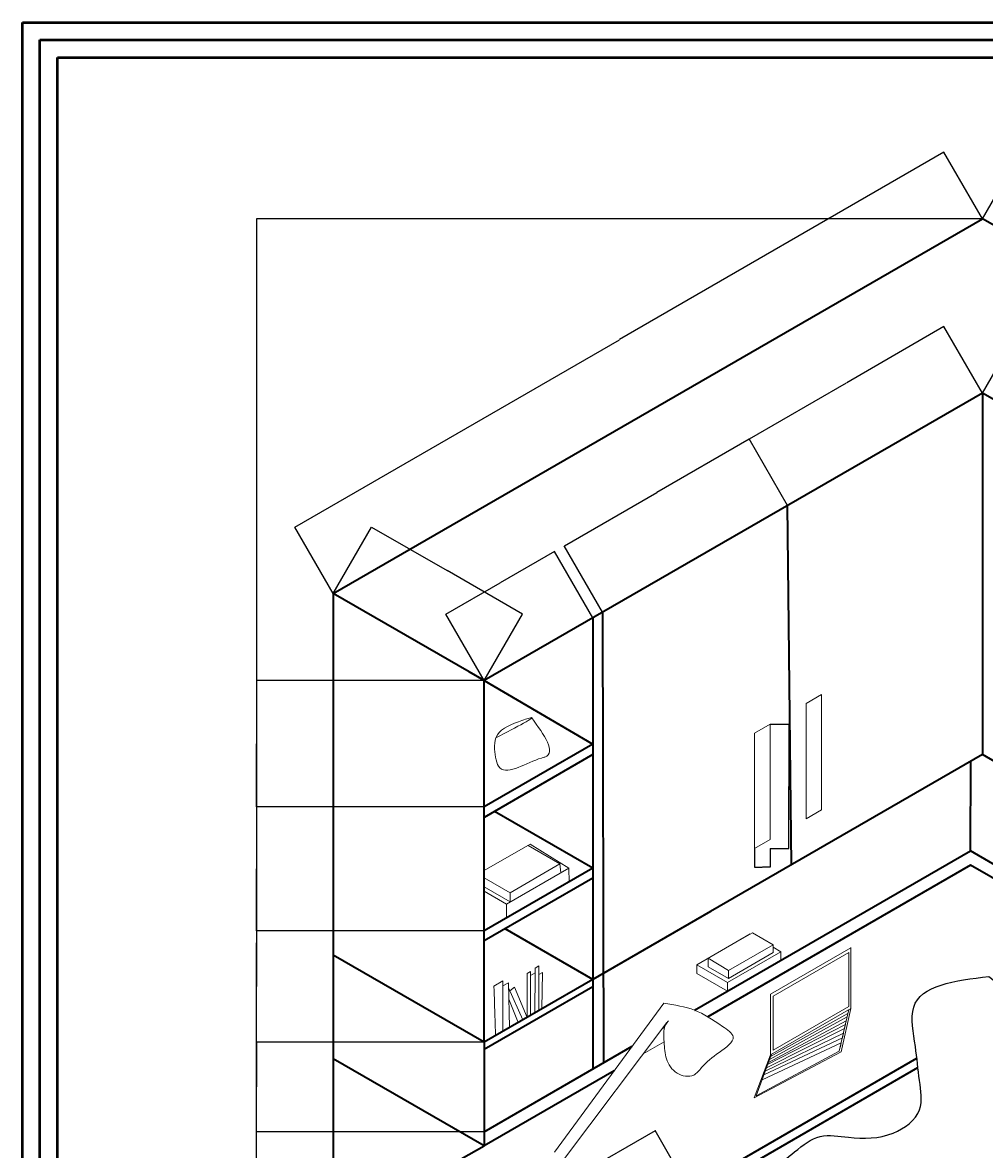
# Model space of a CAD drawing. Units: millimetres. Extents: x -2976 to 8877, y -7187 to 5690.
# Tile 2 of 2: x -2976 to 2542, y -776 to 5690. Entities that reach past the tile are written whole.
import ezdxf

# ---------------------------------------------------------------- set-up
doc = ezdxf.new("R2010")
doc.units = ezdxf.units.MM
doc.header["$MEASUREMENT"] = 0
for name, color, linetype, lineweight in [('A-ANNO-DIMS', 2, 'Continuous', 18), ('A-ANNO-TTLB', 7, 'Continuous', 50), ('A-FURN', 7, 'Continuous', 35), ('A-FURN-ACCS', 3, 'Continuous', 18), ('A-FURN-CHAIR', 4, 'Continuous', 25), ('A-FURN-HDWR', 8, 'Continuous', 18)]:
    doc.layers.add(name, color=color, linetype=linetype, lineweight=lineweight)
doc.styles.get("Standard").update_dxf_attribs({"font": 'arial.ttf'})
doc.dimstyles.get("Standard").update_dxf_attribs({"dimtxt": 0.18, "dimasz": 0.18, "dimexe": 0.18, "dimexo": 0.0625, "dimgap": 0.09, "dimtad": 0, "dimtih": 1, "dimtoh": 1, "dimdec": 0, "dimzin": 0, "dimdsep": 46, "dimtxsty": 'Standard', "dimcen": 0.09, "dimadec": 0, "dimazin": 0, "dimtfac": 1, "dimtdec": 0, "dimtofl": 0, "dimtmove": 0, "dimatfit": 3, "dimfxl": 1, "dimtolj": 1, "dimtzin": 0, "dimarcsym": 0})

# ---------------------------------------------------------------- blocks, each defined once
blk = doc.blocks.new('HANDLE-DOOR-L')
for p, q in [((89.65431383447503, 713.2380158491153), (-0.0001289517056193, 661.4759991724679)), ((89.65431383447503, 51.7624652354541), (89.65431383447503, 713.2380158491153)), ((-0.0001289517058467, 0.0004485588067382), (-0.0001289517058467, 661.4759991724676)), ((-0.0001289517058467, 0.0004485588067382), (89.65431383447503, 51.7624652354541))]:
    blk.add_line(p, q)
blk = doc.blocks.new('*D9')
at = {"layer": 'A-ANNO-DIMS', "color": 0, "lineweight": -2, "transparency": 16777216}
for p, q in [((1313.18315975467, 1663.813910547956), (1420.286294848217, 1663.813910547956)), ((1420.106294848217, 1663.633910547956), (1420.106294848217, 1307.403182837317)), ((1420.106294848217, 950.7563432576469), (1420.106294848217, 1306.987070968286)), ((1313.18315975467, 950.576343257647), (1420.286294848217, 950.576343257647))]:
    blk.add_line(p, q, dxfattribs=at)
at = {"layer": 'A-ANNO-DIMS', "color": 0, "transparency": 16777216}
for points in [[(1420.076294848217, 1663.633910547956), (1420.136294848217, 1663.633910547956), (1420.106294848217, 1663.813910547956)], [(1420.076294848217, 950.7563432576469), (1420.136294848217, 950.7563432576469), (1420.106294848217, 950.576343257647)]]:
    blk.add_solid(points, dxfattribs=at)
at = {"layer": 'Defpoints', "color": 0, "transparency": 16777216}
for p in [(1313.12065975467, 1663.813910547956), (1313.12065975467, 950.576343257647), (1420.106294848217, 950.576343257647)]:
    blk.add_point(p, dxfattribs=at)
at = {"layer": 'A-ANNO-DIMS', "color": 0, "transparency": 16777216, "insert": (1420.106294848217, 1307.195126902801), "char_height": 0.18, "attachment_point": 5}
blk.add_mtext('\\A1;DOOR HANDLE (LEFT) 713 TYP.', dxfattribs=at)
blk = doc.blocks.new('*D10')
at = {"layer": 'A-ANNO-DIMS', "color": 0, "lineweight": -2, "transparency": 16777216}
for p, q in [((1223.466216968489, 950.5138432576465), (1223.466216968489, 843.4107081641002)), ((1313.12065975467, 950.5138432576465), (1313.12065975467, 843.4107081641002)), ((1223.646216968489, 843.5907081641003), (1267.765348320651, 843.5907081641003)), ((1312.94065975467, 843.5907081641003), (1268.821528402507, 843.5907081641003))]:
    blk.add_line(p, q, dxfattribs=at)
at = {"layer": 'A-ANNO-DIMS', "color": 0, "transparency": 16777216}
for points in [[(1223.646216968489, 843.6207081641002), (1223.646216968489, 843.5607081641004), (1223.466216968489, 843.5907081641003)], [(1312.94065975467, 843.6207081641002), (1312.94065975467, 843.5607081641004), (1313.12065975467, 843.5907081641003)]]:
    blk.add_solid(points, dxfattribs=at)
at = {"layer": 'Defpoints', "color": 0, "transparency": 16777216}
for p in [(1223.466216968489, 950.5763432576467), (1313.12065975467, 950.5763432576467), (1223.466216968489, 843.5907081641003)]:
    blk.add_point(p, dxfattribs=at)
at = {"layer": 'A-ANNO-DIMS', "color": 0, "transparency": 16777216, "insert": (1268.293438361579, 843.5907081641003), "char_height": 0.18, "attachment_point": 5}
blk.add_mtext('\\A1;90 TYP.', dxfattribs=at)
blk = doc.blocks.new('*D14')
at = {"layer": 'A-ANNO-DIMS', "color": 0, "lineweight": -2, "transparency": 16777216}
for p, q in [((2530.179259000001, 4564.359981000001), (-1633.847478000003, 4564.359981)), ((-1633.667478000003, 4564.179981), (-1633.667478000002, 411.1110510293304)), ((-1633.667478000001, -3742.321808000003), (-1633.667478000002, 410.7471219706673)), ((-327.7045740000001, -3742.501808000002), (-1633.847478000001, -3742.501808000002))]:
    blk.add_line(p, q, dxfattribs=at)
at = {"layer": 'A-ANNO-DIMS', "color": 0, "transparency": 16777216}
for points in [[(-1633.697478000003, 4564.179981), (-1633.637478000003, 4564.179981), (-1633.667478000003, 4564.359981)], [(-1633.697478000001, -3742.321808000003), (-1633.637478000001, -3742.321808000003), (-1633.667478000001, -3742.501808000002)]]:
    blk.add_solid(points, dxfattribs=at)
at = {"layer": 'Defpoints', "color": 0, "transparency": 16777216}
for p in [(2530.241759000001, 4564.359981000001), (-1633.667478000001, -3742.501808000002), (-327.6420740000001, -3742.501808000002)]:
    blk.add_point(p, dxfattribs=at)
at = {"layer": 'A-ANNO-DIMS', "color": 0, "transparency": 16777216, "insert": (-1633.667478000001, 410.9290864999992), "char_height": 0.18, "attachment_point": 5}
blk.add_mtext('\\A1;8307', dxfattribs=at)
blk = doc.blocks.new('*D16')
at = {"layer": 'A-ANNO-DIMS', "color": 0, "lineweight": -2, "transparency": 16777216}
for p, q in [((-327.7045740000001, 1914.359981000001), (-1633.847478000002, 1914.359981)), ((-1633.667478000002, 1914.179981), (-1633.667478000002, 1552.47832434925)), ((-1633.667478000002, 1190.415931), (-1633.667478000002, 1552.117587650751)), ((-327.7045740000001, 1190.235931), (-1633.847478000001, 1190.235931))]:
    blk.add_line(p, q, dxfattribs=at)
at = {"layer": 'A-ANNO-DIMS', "color": 0, "transparency": 16777216}
for points in [[(-1633.697478000002, 1914.179981), (-1633.637478000002, 1914.179981), (-1633.667478000002, 1914.359981)], [(-1633.697478000001, 1190.415931), (-1633.637478000002, 1190.415931), (-1633.667478000002, 1190.235931)]]:
    blk.add_solid(points, dxfattribs=at)
at = {"layer": 'Defpoints', "color": 0, "transparency": 16777216}
for p in [(-327.6420740000001, 1914.359981000001), (-1633.667478000002, 1190.235931), (-327.6420740000001, 1190.235931)]:
    blk.add_point(p, dxfattribs=at)
at = {"layer": 'A-ANNO-DIMS', "color": 0, "transparency": 16777216, "insert": (-1633.667478000001, 1552.297956), "char_height": 0.18, "attachment_point": 5}
blk.add_mtext('\\A1;724.1', dxfattribs=at)
blk = doc.blocks.new('*D17')
at = {"layer": 'A-ANNO-DIMS', "color": 0, "lineweight": -2, "transparency": 16777216}
for p, q in [((-327.7045740000001, 1190.235931), (-1633.847478000001, 1190.235931)), ((-1633.667478000002, 1190.055931), (-1633.667478000002, 834.1931958492496)), ((-1633.667478000002, 477.9697239999999), (-1633.667478000002, 833.8324591507504)), ((-327.7045740000001, 477.7897240000002), (-1633.847478000001, 477.7897239999999))]:
    blk.add_line(p, q, dxfattribs=at)
at = {"layer": 'A-ANNO-DIMS', "color": 0, "transparency": 16777216}
for points in [[(-1633.697478000002, 1190.055931), (-1633.637478000002, 1190.055931), (-1633.667478000002, 1190.235931)], [(-1633.697478000001, 477.9697239999999), (-1633.637478000002, 477.9697239999999), (-1633.667478000002, 477.7897239999999)]]:
    blk.add_solid(points, dxfattribs=at)
at = {"layer": 'Defpoints', "color": 0, "transparency": 16777216}
for p in [(-327.6420740000001, 1190.235931), (-1633.667478000002, 477.7897239999999), (-327.6420740000001, 477.7897240000002)]:
    blk.add_point(p, dxfattribs=at)
at = {"layer": 'A-ANNO-DIMS', "color": 0, "transparency": 16777216, "insert": (-1633.667478000001, 834.0128275000003), "char_height": 0.18, "attachment_point": 5}
blk.add_mtext('\\A1;712.4', dxfattribs=at)
blk = doc.blocks.new('*D18')
at = {"layer": 'A-ANNO-DIMS', "color": 0, "lineweight": -2, "transparency": 16777216}
for p, q in [((-327.7045740000001, 477.7897240000002), (-1633.847478000002, 477.7897239999999)), ((-1633.667478000002, 477.6097239999999), (-1633.667478000002, 158.9980610293313)), ((-1633.667478000002, -159.9775310000002), (-1633.667478000002, 158.6341319706683)), ((-327.7045740000001, -160.1575310000001), (-1633.847478000002, -160.1575310000002))]:
    blk.add_line(p, q, dxfattribs=at)
at = {"layer": 'A-ANNO-DIMS', "color": 0, "transparency": 16777216}
for points in [[(-1633.697478000002, 477.6097239999999), (-1633.637478000002, 477.6097239999999), (-1633.667478000002, 477.7897239999999)], [(-1633.697478000002, -159.9775310000002), (-1633.637478000002, -159.9775310000002), (-1633.667478000002, -160.1575310000002)]]:
    blk.add_solid(points, dxfattribs=at)
at = {"layer": 'Defpoints', "color": 0, "transparency": 16777216}
for p in [(-327.6420740000001, 477.7897240000002), (-1633.667478000002, -160.1575310000002), (-327.6420740000001, -160.1575310000001)]:
    blk.add_point(p, dxfattribs=at)
at = {"layer": 'A-ANNO-DIMS', "color": 0, "transparency": 16777216, "insert": (-1633.667478000001, 158.8160965000003), "char_height": 0.18, "attachment_point": 5}
blk.add_mtext('\\A1;638', dxfattribs=at)
blk = doc.blocks.new('*D19')
at = {"layer": 'A-ANNO-DIMS', "color": 0, "lineweight": -2, "transparency": 16777216}
for p, q in [((-327.7045740000001, -160.1575310000001), (-1633.847478000002, -160.1575310000002)), ((-1633.667478000002, -160.3375310000003), (-1633.667478000002, -416.6881374706688)), ((-1633.667478000002, -673.4026730000003), (-1633.667478000002, -417.0520665293318)), ((-327.7045740000001, -673.5826730000002), (-1633.847478000001, -673.5826730000003))]:
    blk.add_line(p, q, dxfattribs=at)
at = {"layer": 'A-ANNO-DIMS', "color": 0, "transparency": 16777216}
for points in [[(-1633.697478000002, -160.3375310000003), (-1633.637478000002, -160.3375310000003), (-1633.667478000002, -160.1575310000002)], [(-1633.697478000001, -673.4026730000003), (-1633.637478000002, -673.4026730000003), (-1633.667478000002, -673.5826730000003)]]:
    blk.add_solid(points, dxfattribs=at)
at = {"layer": 'Defpoints', "color": 0, "transparency": 16777216}
for p in [(-327.6420740000001, -160.1575310000001), (-1633.667478000002, -673.5826730000003), (-327.6420740000001, -673.5826730000002)]:
    blk.add_point(p, dxfattribs=at)
at = {"layer": 'A-ANNO-DIMS', "color": 0, "transparency": 16777216, "insert": (-1633.667478000001, -416.8701019999998), "char_height": 0.18, "attachment_point": 5}
blk.add_mtext('\\A1;513.4', dxfattribs=at)
blk = doc.blocks.new('*D24')
at = {"layer": 'A-ANNO-DIMS', "color": 0, "lineweight": -2, "transparency": 16777216}
for p, q in [((652.7837904139722, -667.9703643117301), (52.96397228998472, -1014.276497770886)), ((872.9084249999999, -1048.877415412263), (652.8496749866534, -667.7244797390488)), ((-547.4861894539579, -1360.946560288706), (52.33362867002966, -1014.640426829549)), ((-327.6733239999999, -1742.033611412263), (-547.7320740266391, -1360.880675716025))]:
    blk.add_line(p, q, dxfattribs=at)
at = {"layer": 'A-ANNO-DIMS', "color": 0, "transparency": 16777216}
for points in [[(652.7687904139723, -667.9443835496166), (652.7987904139723, -667.9963450738435), (652.9396749866535, -667.8803643117301)], [(-547.5011894539577, -1360.920579526592), (-547.4711894539579, -1360.972541050819), (-547.6420740266392, -1361.036560288706)]]:
    blk.add_solid(points, dxfattribs=at)
at = {"layer": 'Defpoints', "color": 0, "transparency": 16777216}
for p in [(652.9396749866535, -667.8803643117301), (872.9396749999999, -1048.931542), (-327.6420739999999, -1742.087737999999)]:
    blk.add_point(p, dxfattribs=at)
at = {"layer": 'A-ANNO-DIMS', "color": 0, "transparency": 16777216, "insert": (52.64880048000714, -1014.458462300218), "char_height": 0.18, "attachment_point": 5}
blk.add_mtext('\\A1;1386.3', dxfattribs=at)
blk = doc.blocks.new('*D25')
at = {"layer": 'A-ANNO-DIMS', "color": 0, "lineweight": -2, "transparency": 16777216}
for p, q in [((2310.085874749474, 4945.321158107162), (448.6023127229957, 3870.593122479113)), ((2530.210509, 4564.414107587736), (2310.151759322155, 4945.567042679844)), ((-1413.511592923435, 2795.501157792401), (447.9719691030407, 3870.22919342045)), ((-1193.698728, 2414.414107587737), (-1413.757477496116, 2795.567042365082))]:
    blk.add_line(p, q, dxfattribs=at)
at = {"layer": 'A-ANNO-DIMS', "color": 0, "transparency": 16777216}
for points in [[(2310.070874749474, 4945.347138869276), (2310.100874749474, 4945.295177345049), (2310.241759322155, 4945.411158107162)], [(-1413.526592923435, 2795.527138554515), (-1413.496592923435, 2795.475177030287), (-1413.667477496116, 2795.411157792401)]]:
    blk.add_solid(points, dxfattribs=at)
at = {"layer": 'Defpoints', "color": 0, "transparency": 16777216}
for p in [(2310.241759322155, 4945.411158107162), (2530.241759, 4564.359980999999), (-1193.667478, 2414.359981)]:
    blk.add_point(p, dxfattribs=at)
at = {"layer": 'A-ANNO-DIMS', "color": 0, "transparency": 16777216, "insert": (448.2871409130193, 3870.411157949782), "char_height": 0.18, "attachment_point": 5}
blk.add_mtext('\\A1;4300', dxfattribs=at)
blk = doc.blocks.new('*D26')
at = {"layer": 'A-ANNO-DIMS', "color": 0, "lineweight": -2, "transparency": 16777216}
for p, q in [((2530.273009, 4564.414107587735), (2750.331758610178, 4945.567042562642)), ((2750.397643182859, 4945.321157989961), (5131.496553235272, 3570.593061304077)), ((7513.225594241101, 2195.501158342615), (5132.126684188691, 3570.229255028497)), ((7293.412728999999, 1814.414107587736), (7513.471478813783, 2195.567042915297))]:
    blk.add_line(p, q, dxfattribs=at)
at = {"layer": 'A-ANNO-DIMS', "color": 0, "transparency": 16777216}
for points in [[(2750.412643182859, 4945.347138752074), (2750.382643182859, 4945.295177227848), (2750.241758610178, 4945.411157989961)], [(7513.240594241101, 2195.527139104729), (7513.210594241101, 2195.475177580502), (7513.381478813783, 2195.411158342615)]]:
    blk.add_solid(points, dxfattribs=at)
at = {"layer": 'Defpoints', "color": 0, "transparency": 16777216}
for p in [(2530.241759, 4564.359980999999), (7513.381478813783, 2195.411158342615), (7293.381479, 1814.359981)]:
    blk.add_point(p, dxfattribs=at)
at = {"layer": 'A-ANNO-DIMS', "color": 0, "transparency": 16777216, "insert": (5131.81161871198, 3570.411158166288), "char_height": 0.18, "attachment_point": 5}
blk.add_mtext('\\A1;5500', dxfattribs=at)
blk = doc.blocks.new('*D28')
at = {"layer": 'A-ANNO-DIMS', "color": 0, "lineweight": -2, "transparency": 16777216}
for p, q in [((-1193.636227999999, 2414.414107587737), (-973.5774782610742, 2795.567042785639)), ((-973.5115936883936, 2795.321158212958), (-540.9698417647282, 2545.593061304078)), ((-107.7979588876464, 2295.501158119617), (-540.3397108113113, 2545.229255028497)), ((-327.610824, 1914.414107587736), (-107.5520743149651, 2295.567042692298))]:
    blk.add_line(p, q, dxfattribs=at)
at = {"layer": 'A-ANNO-DIMS', "color": 0, "transparency": 16777216}
for points in [[(-973.4965936883935, 2795.347138975071), (-973.5265936883935, 2795.295177450845), (-973.6674782610744, 2795.411158212958)], [(-107.7829588876465, 2295.52713888173), (-107.8129588876464, 2295.475177357504), (-107.6420743149651, 2295.411158119617)]]:
    blk.add_solid(points, dxfattribs=at)
at = {"layer": 'Defpoints', "color": 0, "transparency": 16777216}
for p in [(-1193.667477999999, 2414.359981), (-107.6420743149651, 2295.411158119617), (-327.642074, 1914.359981)]:
    blk.add_point(p, dxfattribs=at)
at = {"layer": 'A-ANNO-DIMS', "color": 0, "transparency": 16777216, "insert": (-540.65477628802, 2545.411158166288), "char_height": 0.18, "attachment_point": 5}
blk.add_mtext('\\A1;1000', dxfattribs=at)
blk = doc.blocks.new('*D30')
at = {"layer": 'A-ANNO-DIMS', "color": 0, "lineweight": -2, "transparency": 16777216}
for p, q in [((76.27645158373389, 2655.630686394234), (-235.2898032352716, 2475.747825304078)), ((296.401086, 2274.723635587736), (76.34233615641529, 2655.876570966916)), ((-547.486189007694, 2295.501157938343), (-235.9199341886884, 2475.384019028498)), ((-327.6733239999999, 1914.414107587736), (-547.732073580375, 2295.567042511024))]:
    blk.add_line(p, q, dxfattribs=at)
at = {"layer": 'A-ANNO-DIMS', "color": 0, "transparency": 16777216}
for points in [[(76.26145158373379, 2655.656667156348), (76.29145158373399, 2655.604705632121), (76.4323361564152, 2655.720686394234)], [(-547.501189007694, 2295.527138700456), (-547.4711890076939, 2295.475177176228), (-547.642073580375, 2295.411157938342)]]:
    blk.add_solid(points, dxfattribs=at)
at = {"layer": 'Defpoints', "color": 0, "transparency": 16777216}
for p in [(76.4323361564152, 2655.720686394234), (296.432336, 2274.669509), (-327.6420739999999, 1914.359981)]:
    blk.add_point(p, dxfattribs=at)
at = {"layer": 'A-ANNO-DIMS', "color": 0, "transparency": 16777216, "insert": (-235.6048687119801, 2475.565922166288), "char_height": 0.18, "attachment_point": 5}
blk.add_mtext('\\A1;720.6', dxfattribs=at)
blk = doc.blocks.new('*D31')
at = {"layer": 'A-ANNO-DIMS', "color": 0, "lineweight": -2, "transparency": 16777216}
for p, q in [((1193.11868536768, 3300.439851768452), (662.9351433317158, 2994.338241054078)), ((1413.24332, 2919.532800587737), (1193.184569940361, 3300.685736341132)), ((132.1214703423352, 2687.872824064124), (662.3050123782991, 2993.974434778498)), ((351.9343360000001, 2306.785772587737), (131.875585769654, 2687.938708636805))]:
    blk.add_line(p, q, dxfattribs=at)
at = {"layer": 'A-ANNO-DIMS', "color": 0, "transparency": 16777216}
for points in [[(1193.10368536768, 3300.465832530565), (1193.13368536768, 3300.413871006337), (1193.274569940361, 3300.529851768451)], [(132.1064703423351, 2687.898804826238), (132.1364703423353, 2687.846843302011), (131.9655857696539, 2687.782824064124)]]:
    blk.add_solid(points, dxfattribs=at)
at = {"layer": 'Defpoints', "color": 0, "transparency": 16777216}
for p in [(1193.274569940361, 3300.529851768451), (1413.27457, 2919.478674), (351.965586, 2306.731646)]:
    blk.add_point(p, dxfattribs=at)
at = {"layer": 'A-ANNO-DIMS', "color": 0, "transparency": 16777216, "insert": (662.6200778550075, 2994.156337916288), "char_height": 0.18, "attachment_point": 5}
blk.add_mtext('\\A1;1225.5', dxfattribs=at)
blk = doc.blocks.new('*D32')
at = {"layer": 'A-ANNO-DIMS', "color": 0, "lineweight": -2, "transparency": 16777216}
for p, q in [((2310.08587432076, 3945.321158849719), (1752.073229923222, 3623.152408395585)), ((2530.210509, 3564.414107587737), (2310.151758893441, 3945.567043422399)), ((1193.430454572267, 3300.619851665871), (1751.443098969805, 3622.788602120005)), ((1413.24332, 2919.532800587737), (1193.184569999585, 3300.685736238552))]:
    blk.add_line(p, q, dxfattribs=at)
at = {"layer": 'A-ANNO-DIMS', "color": 0, "transparency": 16777216}
for points in [[(2310.07087432076, 3945.347139611832), (2310.10087432076, 3945.295178087604), (2310.241758893441, 3945.411158849719)], [(1193.415454572267, 3300.645832427985), (1193.445454572267, 3300.593870903757), (1193.274569999585, 3300.529851665871)]]:
    blk.add_solid(points, dxfattribs=at)
at = {"layer": 'Defpoints', "color": 0, "transparency": 16777216}
for p in [(2310.241758893441, 3945.411158849719), (2530.241759, 3564.359981), (1413.27457, 2919.478674)]:
    blk.add_point(p, dxfattribs=at)
at = {"layer": 'A-ANNO-DIMS', "color": 0, "transparency": 16777216, "insert": (1751.758164446514, 3622.970505257795), "char_height": 0.18, "attachment_point": 5}
blk.add_mtext('\\A1;1289.8', dxfattribs=at)
blk = doc.blocks.new('*D33')
at = {"layer": 'A-ANNO-DIMS', "color": 0, "lineweight": -2, "transparency": 16777216}
for p, q in [((2530.273009, 3564.414107587737), (2750.331758502398, 3945.567042375962)), ((2750.397643075079, 3945.321157803281), (3399.445745610272, 3570.593061087572)), ((4049.123979098881, 3195.501158096283), (3400.075876563688, 3570.229254811992)), ((3829.311114, 2814.414107587736), (4049.369863671563, 3195.567042668964))]:
    blk.add_line(p, q, dxfattribs=at)
at = {"layer": 'A-ANNO-DIMS', "color": 0, "transparency": 16777216}
for points in [[(2750.412643075078, 3945.347138565394), (2750.382643075079, 3945.295177041167), (2750.241758502398, 3945.411157803281)], [(4049.138979098881, 3195.527138858396), (4049.108979098881, 3195.47517733417), (4049.279863671563, 3195.411158096283)]]:
    blk.add_solid(points, dxfattribs=at)
at = {"layer": 'Defpoints', "color": 0, "transparency": 16777216}
for p in [(2530.241759, 3564.359981000001), (4049.279863671563, 3195.411158096283), (3829.279864, 2814.359981)]:
    blk.add_point(p, dxfattribs=at)
at = {"layer": 'A-ANNO-DIMS', "color": 0, "transparency": 16777216, "insert": (3399.76081108698, 3570.411157949782), "char_height": 0.18, "attachment_point": 5}
blk.add_mtext('\\A1;1500', dxfattribs=at)

msp = doc.modelspace()

# ---------------------------------------------------------------- linework, layer by layer
at = {"layer": 'A-ANNO-TTLB'}
for points in [[(-2976.020185178524, 5689.883775799608), (8877.112005194242, 5689.883775799608), (8877.112005194242, -5692.972772104557), (-2976.020185178524, -5692.972772104557)], [(-2876.020185178524, 5589.883775799608), (8777.112005194242, 5589.883775799608), (8777.112005194242, -5592.972772104559), (-2876.020185178524, -5592.972772104556)], [(-2776.020185178524, 5489.883775799608), (8677.112005194242, 5489.883775799608), (8677.112005194242, -5492.972772104557), (-2776.020185178524, -5492.972772104557)]]:
    msp.add_lwpolyline(points, close=True, dxfattribs=at)
at = {"layer": 'A-FURN'}
for p, q in [((-1193.66747761529, 2414.359980599719), (2530.241758657795, 4564.359980599717)), ((3396.267162442234, 4064.359980599718), (2530.241758657796, 4564.359980599717)), ((2530.241758657797, 3564.359980599719), (-327.642073830851, 1914.359980599719)), ((3396.267162442236, 3064.359980599719), (2530.241758657797, 3564.359980599719)), ((2530.241758657797, 3564.359980599719), (2530.241758657797, 1489.842468911971)), ((1436.038522596671, 858.10393602392), (1413.274570085147, 2919.47867360132)), ((-414.244614209295, 1964.359980599719), (-1193.66747761529, 2414.359980599719)), ((-1193.66747761529, 2414.359980599719), (-1193.66747761529, 339.8424689119711)), ((296.4323356883124, 2274.669508929964), (296.4323356883124, -313.2731446386687)), ((351.9655863579701, 2306.731646153066), (357.7042903155056, -277.8977651408841)), ((-327.6420738308511, 1914.359980599719), (-414.244614209295, 1964.359980599719)), ((-327.642073830851, -160.157531088029), (-327.642073830851, 1914.359980599719)), ((-327.6420738308511, 1914.359980599719), (296.4323356883124, 1550.545459165092)), ((296.4323356883124, 1550.545459165092), (-327.642073830851, 1190.235930834846)), ((296.4323356883124, 1489.834783541912), (-327.642073830851, 1129.525255211666)), ((2530.241758657797, 1489.842468911971), (971.396031845807, 589.8424689119709)), ((5128.317970011113, -10.1575310880287), (2530.241758657797, 1489.842468911971)), ((2461.912680004405, 936.9675150770707), (2463.245552934603, 1451.162191503001)), ((296.4323356883124, 838.0992527328634), (-267.9871905412595, 1163.967018137388)), ((879.4057281996977, 23.30670045816885), (2461.912680004405, 936.9675150770703)), ((5128.317970011113, -602.482296876944), (2461.912680004405, 936.9675150770705)), ((2462.198248141479, 855.963524743986), (954.6291691149065, -14.43188885396103)), ((5128.317970011113, -683.3214143692167), (2462.198248141479, 855.963524743986)), ((296.4323356883124, 838.0992527328634), (-327.642073830851, 477.7897244026179)), ((296.4323356883124, 780.9903520272346), (-327.642073830851, 420.6808236969889)), ((971.396031845807, 589.8424689119709), (884.7934914673631, 539.8424689119709)), ((884.7934914673631, 539.8424689119709), (296.4323356883124, 200.1519972422166)), ((296.4323356883124, 200.1519972422165), (-206.5884350478719, 490.5711746347257)), ((-327.642073830851, -160.157531088029), (-1193.66747761529, 339.842468911971)), ((-1193.66747761529, 339.8424689119711), (-1193.66747761529, -254.7515361428099)), ((296.4323356883124, 200.1519972422165), (-327.642073830851, -160.1575310880289)), ((296.4323356883124, 158.2003521335282), (-327.642073830851, -202.1091761967174)), ((-327.642073830851, -160.157531088029), (-327.642073830851, -754.7515361428099)), ((-327.642073830851, -673.5826729689143), (520.823438857581, -183.7208808201343)), ((-327.642073830851, -754.7515361428101), (-1193.66747761529, -254.75153614281)), ((-1193.66747761529, -254.7515361428099), (-1193.66747761529, -1242.087737987627)), ((-376.8059096461261, -1713.702984145284), (2154.739901078788, -252.1143288573858)), ((-327.6420738308511, -1742.087737987627), (2160.78160776331, -305.3956555613991)), ((417.3596522714476, -324.624589030912), (-327.6420738308511, -754.7515361428101)), ((-1193.66747761529, -1242.087737987628), (-327.642073830851, -754.7515361428099))]:
    msp.add_line(p, q, dxfattribs=at)
at = {"layer": 'A-FURN-ACCS'}
for p, q in [((-327.642073830851, 823.9862566569846), (-63.67221271804601, 976.3893270284107)), ((-63.67221271804601, 976.3893270284107), (157.9890071967675, 838.476890398736)), ((106.5181614221328, 863.6441505227884), (-76.2172126559859, 969.1464679372572)), ((-177.7092646844576, 696.7822340564073), (106.5181614221328, 863.644150522788)), ((112.2130167183177, 812.0481099735814), (106.5181614221328, 863.6441505227884)), ((-177.7092646844576, 696.7822340564073), (-327.642073830851, 783.3459817774341)), ((-199.3837496253893, 632.1476330464252), (157.9890071967675, 838.476890398736)), ((112.2130167183177, 812.0481099735814), (112.2130167183177, 812.0481099735814)), ((157.9890071967675, 838.476890398736), (158.9140195003065, 758.7030158632142)), ((-177.7092646844576, 644.6614027616187), (-327.642073830851, 731.2251504826456)), ((-199.3837496253893, 632.1476330464252), (-327.642073830851, 706.1976110522586)), ((-177.7092646844576, 644.6614027616187), (-177.7092646844576, 696.7822340564073)), ((-199.3837496253893, 551.8397024084514), (-199.3837496253893, 632.1476330464252)), ((891.6966553506207, 283.4701452138065), (1198.477232587903, 460.5899940639003)), ((1211.253469687948, 467.9663579928415), (957.3538366640404, 321.3773365193415)), ((1330.426950857538, 399.1615165593146), (1211.253469687948, 467.9663579928415)), ((1330.426950857538, 399.1615165593146), (1073.771553798695, 250.9814539784213)), ((1330.426950857538, 353.8911661544221), (1330.426950857538, 399.1615165593146)), ((1067.737300610673, 181.8330312845996), (1374.517877847956, 358.9528801346935)), ((1073.771553798695, 205.7111035735288), (1330.426950857538, 353.8911661544221)), ((1314.477737066365, 114.6747498336772), (1775.586664088565, 380.896112975684)), ((1763.339210141246, 354.2973124109074), (1329.796176381467, 103.9911251644123)), ((1374.517877847956, 358.9528801346935), (1330.426950857538, 384.4087887014314)), ((1374.517877847956, 358.9528801346935), (1374.517877847956, 309.1598333366452)), ((1763.339210141246, 44.97321932032673), (1763.339210141246, 354.2973124109074)), ((1775.586664088565, 33.96266293645363), (1775.586664088565, 382.4441532261553)), ((-35.70989695761819, 264.8460628584887), (-13.68269883398375, 277.5634716246623)), ((-35.70989695761819, 238.3080850810973), (-35.70989695761819, 264.8460628584887)), ((-13.68269883398375, 277.5634716246623), (-13.68269883398375, 21.10699858101888)), ((1067.737300610673, 181.8330312845996), (891.6966553506207, 283.4701452138065)), ((891.6966553506207, 283.4701452138065), (891.6966553506207, 233.6770984157585)), ((1073.771553798695, 250.9814539784213), (957.3538366640404, 321.3773365193415)), ((957.3538366640404, 321.3773365193415), (957.3538366640404, 272.9249038996634)), ((1073.771553798695, 205.7111035735288), (957.3538366640406, 272.9249038996634)), ((-81.4882993160054, 233.5734420086869), (-62.06782334018498, 244.7858590411174)), ((-81.4882993160054, -18.04058310984055), (-81.4882993160054, 233.5734420086869)), ((-62.06782334018498, 244.7858590411174), (-61.119136439371, -6.280441439848232)), ((-61.98602239539514, 223.1375569863364), (-35.70989695761819, 238.3080850810973)), ((-35.70989695761819, 238.3080850810973), (-37.67707321873741, 7.253840070944761)), ((-13.68269883398375, 228.0265917678335), (7.407007671106839, 240.2027394956776)), ((7.407007671106839, 240.2027394956776), (3.8865255356136, 31.25059500025896)), ((1067.737300610673, 132.0399844865514), (891.6966553506207, 233.6770984157584)), ((1073.771553798695, 205.7111035735288), (1073.771553798695, 250.9814539784213)), ((-220.4101767781931, 191.3449773678665), (-271.5520290960126, 161.8182151653172)), ((-271.5520290960126, 161.8182151653172), (-270.7661164541205, 135.1150718135613)), ((-270.7661164541205, 135.1150718135613), (-266.7339577728417, -1.886556031473446)), ((-220.4101767781931, -98.24716645896272), (-220.4101767781931, 191.3449773678665)), ((-220.4101767781931, 162.3139186864136), (-189.1168065430538, 180.3811544155219)), ((-189.1168065430538, 180.3811544155219), (-182.1723087574528, -76.17052306395101)), ((-188.3541545387434, 152.2063810799184), (-105.7698926018756, -32.05956752979068)), ((-180.5793088352652, 134.8587740995383), (-153.8780467145843, 156.0431597807182)), ((-153.8780467145843, 156.0431597807182), (-81.4882993160054, -18.04058310984055)), ((1067.737300610673, 132.0399844865514), (1067.737300610673, 181.8330312845996)), ((-186.5709807983657, 86.33031221864195), (-132.3420158813715, -47.40099005814761)), ((1314.477737066365, 114.6747498336772), (1314.477737066365, -232.2587002055529)), ((1329.796176381467, 103.9911251644123), (1329.796176381467, 100.0068002701009)), ((1329.796176381467, 100.0068002701009), (1329.796176381467, -205.3329679261686)), ((74.7991430560337, -791.1457519195437), (702.1545995256746, 63.22767765958269)), ((1314.477737066365, -232.2587002055529), (1775.586664088565, 33.96266293645363)), ((1315.698573881739, -242.2822918999594), (1759.010602918231, 3.478565645292746)), ((1329.796176381467, -205.3329679261686), (1763.339210141246, 44.97321932032673)), ((1764.519677161382, 27.5731350549263), (1709.643093137357, -212.4359126311652)), ((1775.586664088565, 33.96266293645363), (1720.06111694552, -216.2336867356489)), ((-266.7339577728417, -1.886556031473446), (-265.5194323906064, -43.15277781929274)), ((-265.5194323906064, -43.15277781929274), (-263.1713152174059, -122.935321247697)), ((-124.83062786904, -43.0642881672403), (-86.7091573347111, -21.05484689234106)), ((720.8745203412259, -47.45045240482432), (132.6519606441791, -828.0224899209036)), ((1298.454207517327, -288.9249767934649), (1745.004231702682, -57.77990874353168)), ((1749.554845574504, -37.87727593233331), (1302.986800983088, -276.6651857227927)), ((1309.574107340288, -258.8477925972352), (1754.657668487373, -15.55949340978225)), ((1745.004231702682, -57.77990874353168), (1739.547320137298, -81.64633868643091)), ((1754.657668487373, -15.55949340978225), (1749.554845574504, -37.87727593233331)), ((-263.1713152174059, -122.935321247697), (-220.4101767781931, -98.24716645896272)), ((-182.1723087574528, -76.17052306395101), (-220.4101767781931, -98.24716645896272)), ((693.1671140616588, -84.21821354793072), (707.4782294176518, -75.95568724474428)), ((1284.59896092048, -326.4007464148008), (1733.558319410818, -107.8399217331561)), ((1739.547320137298, -81.64633868643091), (1291.54722155121, -307.6070416008066)), ((1733.558319410818, -107.8399217331561), (1727.378830032197, -134.8666287945865)), ((704.2608128081919, -158.9821267642068), (584.8915677094249, -227.8999925549423)), ((1266.20490955538, -376.1531074820013), (1720.732036574584, -163.9371439569243)), ((1727.378830032197, -134.8666287945865), (1276.642333586852, -347.9218886646732)), ((1720.732036574584, -163.9371439569243), (1715.465837659967, -186.9694702013817)), ((1221.897540749167, -479.7465289758547), (1720.06111694552, -216.2336867356489)), ((1314.477737066365, -232.2587002055529), (1221.897540749167, -479.7465289758547)), ((1232.543244990366, -467.2014174121968), (1709.643093137357, -212.4359126311653)), ((1320.741422183339, -228.6423599171493), (1232.543244990366, -467.2014174121971)), ((1291.54722155121, -307.6070416008066), (1284.59896092048, -326.4007464148008)), ((1302.986800983088, -276.6651857227927), (1298.454207517327, -288.9249767934649)), ((1276.642333586852, -347.9218886646732), (1266.20490955538, -376.1531074820013))]:
    msp.add_line(p, q, dxfattribs=at)
for points, knots in [([(-260.293606793407, 1586.748621185348), (-141.162942500993, 1647.994484860027), (15.63941887566356, 1728.607617555821), (-167.0849617852662, 1667.768432429077), (-264.5043083032038, 1621.986886855783), (-270.750528452702, 1507.670459406595), (-241.1502316043307, 1334.418395447162), (-73.78982100906667, 1452.336140702227), (94.46400125543995, 1492.607973846043), (16.39438488570566, 1601.509328459258), (-55.1080281468976, 1701.249918966154)], [0, 0, 0, 0, 228.4221037547296, 300.6541218594215, 459.1553973139077, 524.6500273746647, 636.3104016164775, 880.2858352928639, 902.1307042600284, 1139.973323613984, 1139.973323613984, 1139.973323613984, 1139.973323613984]), ([(702.1545995256746, 63.22767765958269), (763.9983754123859, 53.56600421413238), (888.779960028105, 34.07173975053658), (1001.213230100055, -44.95840502425531), (1139.638614330902, -136.66957126607), (1004.921334435568, -227.4311203582509), (935.1113904244526, -283.4802922830645), (871.5422803895792, -366.9406826496664), (766.871898985401, -348.179196501972), (709.9884391744682, -258.2680763795186), (704.3224902704835, -156.0478454114954), (698.5266948006233, -71.54578622784004), (726.8697443910802, -40.15171438486034), (729.5676099824476, -37.16343375091572)], [0, 0, 0, 0, 181.6910758317479, 366.5963151142557, 452.5814190780727, 572.4075296191207, 705.69394738291, 767.5177883897458, 863.4693651047227, 965.681190749868, 1063.506464783338, 1177.564126407045, 1189.56295787331, 1189.56295787331, 1189.56295787331, 1189.56295787331])]:
    msp.add_open_spline(points, degree=3, knots=knots, dxfattribs=at)
at = {"layer": 'A-FURN-CHAIR'}
msp.add_open_spline([(2567.327213554687, 217.3777815164612), (2371.604006962237, 192.7327323130228), (2081.31339379434, 156.1799567409558), (2150.139936282865, -182.4667104222866), (2165.116014388808, -365.952377867469), (2201.134482322425, -570.5848202688835), (2001.966179159994, -713.9202466194699), (1796.942794050407, -716.3269363524186), (1590.45379523456, -678.4075351907952), (1425.098437734223, -813.6407202142198), (1195.207760947901, -994.0076673186782), (1334.194099928929, -1211.943894338208), (1433.600624954212, -1310.666009676965), (1490.614413886304, -1345.956672059368), (1614.157571527384, -1391.232703225471), (1813.084480556488, -1488.982700143385), (2144.550172737321, -1441.760630520553), (2511.026644645633, -1393.796613114915), (2787.65137241148, -1067.523731355003), (2900.240674189164, -675.4125804627595), (2869.868896878056, -301.0233351137475), (2802.881672971835, 19.87963263450726), (2647.650590440668, 150.0314944362605), (2567.327213554687, 217.3777815164612)], degree=3, knots=[0, 0, 0, 0, 465.8253811586821, 690.8978137033012, 888.5150348665003, 1055.970420950123, 1257.901159625074, 1514.322789017122, 1677.169158812602, 1848.867129305455, 2138.548569140127, 2410.457651988302, 2465.321249117196, 2565.415027162817, 2606.552378177621, 2860.949289062645, 3210.570075939517, 3586.794658316177, 3928.74340176956, 4419.123148240912, 4773.689233456088, 5058.287964198188, 5363.462590944195, 5363.462590944195, 5363.462590944195, 5363.462590944195], dxfattribs=at)

# ---------------------------------------------------------------- block references
at = {"layer": 'A-FURN-HDWR'}
msp.add_blockref('HANDLE-DOOR-L', (1518.679, 1121.017), dxfattribs=at)
at = {"layer": 'A-FURN-HDWR', "rotation": 180}
msp.add_blockref('HANDLE-DOOR-L', (1313.120530802964, 1663.814359106762), dxfattribs=at)

# ---------------------------------------------------------------- dimensions: what is measured, and where the dimension line sits
at = {"layer": 'A-ANNO-DIMS'}
for base, p1, p2, angle, override, picture, middle in [((2310.241759322155, 4945.411158107162), (-1193.667478, 2414.359981), (2530.241759, 4564.359980999999), 30, {"dimdec": 0, "dimlfac": 1, "dimrnd": 0, "dimzin": 0, "dimdsep": 46, "dimlunit": 2}, '*D25', (448.2871409130193, 3870.411157949782)), ((7513.381478813783, 2195.411158342615), (2530.241759, 4564.359980999999), (7293.381479, 1814.359981), 330.0000000000001, {"dimdec": 0, "dimlfac": 1, "dimrnd": 0, "dimzin": 0, "dimdsep": 46, "dimlunit": 2}, '*D26', (5131.81161871198, 3570.411158166288)), ((-1633.667478000001, -3742.501808000002), (2530.241759, 4564.359980999999), (-327.642074, -3742.501808), 90, {"dimdec": 0, "dimlfac": 1, "dimrnd": 0, "dimzin": 0, "dimdsep": 46, "dimlunit": 2}, '*D14', (-1633.667478000001, 410.9290864999992)), ((2310.241758893441, 3945.411158849719), (1413.27457, 2919.478674), (2530.241759, 3564.359981000001), 30, {"dimdec": 1, "dimlfac": 1, "dimrnd": 0, "dimzin": 0, "dimdsep": 46, "dimlunit": 2}, '*D32', (1751.758164446514, 3622.970505257795)), ((4049.279863671563, 3195.411158096283), (2530.241759, 3564.359981000001), (3829.279864, 2814.359981), 330.0000000000001, {"dimdec": 0, "dimlfac": 1, "dimrnd": 0, "dimzin": 0, "dimdsep": 46, "dimlunit": 2}, '*D33', (3399.76081108698, 3570.411157949782)), ((1193.274569940361, 3300.529851768451), (351.965586, 2306.731646), (1413.27457, 2919.478674), 30.00000000000003, {"dimdec": 1, "dimlfac": 1, "dimrnd": 0, "dimzin": 0, "dimdsep": 46, "dimlunit": 2}, '*D31', (662.6200778550075, 2994.156337916288)), ((-107.6420743149651, 2295.411158119617), (-1193.667478, 2414.359981), (-327.642074, 1914.359981), 330, {"dimdec": 0, "dimlfac": 1, "dimrnd": 0, "dimzin": 0, "dimdsep": 46, "dimlunit": 2}, '*D28', (-540.65477628802, 2545.411158166288)), ((76.4323361564152, 2655.720686394234), (-327.642074, 1914.359981), (296.432336, 2274.669509), 29.99999999999996, {"dimdec": 1, "dimlfac": 1, "dimrnd": 0, "dimzin": 0, "dimdsep": 46, "dimlunit": 2}, '*D30', (-235.6048687119801, 2475.565922166288)), ((-1633.667478000002, 1190.235931), (-327.642074, 1914.359981), (-327.642074, 1190.235931), 90, {"dimdec": 1, "dimlfac": 1, "dimrnd": 0, "dimzin": 0, "dimdsep": 46, "dimlunit": 2}, '*D16', (-1633.667478000001, 1552.297956)), ((-1633.667478000002, 477.7897239999999), (-327.642074, 1190.235931), (-327.642074, 477.7897239999999), 90, {"dimdec": 1, "dimlfac": 1, "dimrnd": 0, "dimzin": 0, "dimdsep": 46, "dimlunit": 2}, '*D17', (-1633.667478000001, 834.0128275000003)), ((-1633.667478000002, -160.1575310000002), (-327.642074, 477.7897239999999), (-327.642074, -160.157531), 90, {"dimdec": 0, "dimlfac": 1, "dimrnd": 0, "dimzin": 0, "dimdsep": 46, "dimlunit": 2}, '*D18', (-1633.667478000001, 158.8160965000003)), ((-1633.667478000002, -673.5826730000003), (-327.642074, -160.157531), (-327.642074, -673.582673), 90, {"dimdec": 1, "dimlfac": 1, "dimrnd": 0, "dimzin": 0, "dimdsep": 46, "dimlunit": 2}, '*D19', (-1633.667478000001, -416.8701019999998)), ((652.9396749866535, -667.8803643117301), (-327.642074, -1742.087738), (872.9396749999999, -1048.931542), 29.99999999999999, {"dimdec": 1, "dimlfac": 1, "dimrnd": 0, "dimzin": 0, "dimdsep": 46, "dimlunit": 2}, '*D24', (52.64880048000714, -1014.458462300218))]:
    dim = msp.add_linear_dim(base=base, p1=p1, p2=p2, angle=angle, dimstyle='Standard', override=override, dxfattribs=at)
    dim.commit()
    dim.dimension.update_dxf_attribs({"geometry": picture, "text_midpoint": middle})
for base, p1, p2, angle, text, picture, middle in [((1420.106294848217, 950.576343257647), (1313.12065975467, 1663.813910547955), (1313.12065975467, 950.5763432576467), 270, 'DOOR HANDLE (LEFT) <> TYP.', '*D9', (1420.106294848217, 1307.195126902801)), ((1223.466216968489, 843.5907081641003), (1313.12065975467, 950.5763432576467), (1223.466216968489, 950.5763432576467), 180, '<> TYP.', '*D10', (1268.293438361579, 843.5907081641003))]:
    dim = msp.add_linear_dim(base=base, p1=p1, p2=p2, angle=angle, text=text, dimstyle='Standard', override={"dimdec": 0, "dimlfac": 1, "dimrnd": 0, "dimzin": 0, "dimdsep": 46, "dimlunit": 2}, dxfattribs=at)
    dim.commit()
    dim.dimension.update_dxf_attribs({"geometry": picture, "text_midpoint": middle})

doc.saveas('drawing.dxf')
